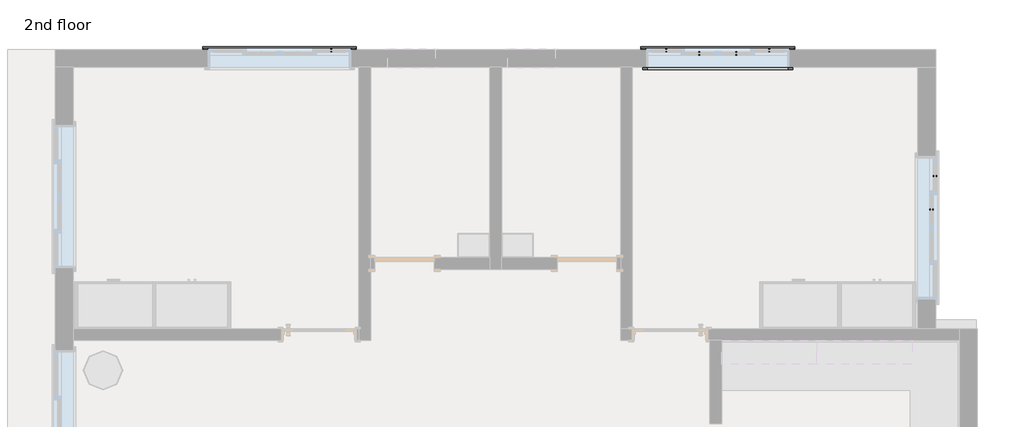
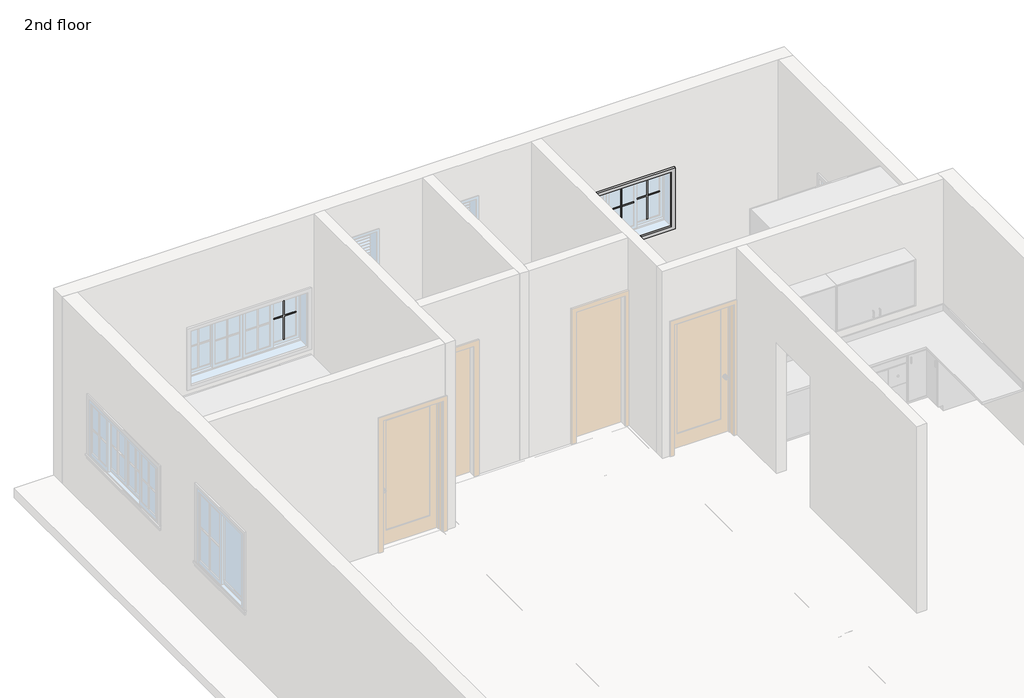
# One storey, part 4 of 4: 10 proxies.
"""IFC4 building model written with IfcOpenShell, lengths in millimetres."""

from ifc_helpers import new_model, si_unit, origin, place, context, project, spatial, transform, mapped, element, save
from components import muntin_pattern_2x2_muntin_pattern_2x2_31a16349, trim_window_exterior_flat_with_sill_3c945769, trim_window_interior_flat_picture_frame_0edfbaa2

model = new_model("IFC4")

# Units and contexts
model_context = context("Model", 3, world=origin())
ifc_project = project(units=[si_unit("LENGTHUNIT", "METRE", prefix="MILLI")], contexts=[model_context])

# Site, building, storey
site = spatial("IfcSite", under=ifc_project)
building = spatial("IfcBuilding", under=site)
storey = spatial("IfcBuildingStorey", under=building, Name="2nd floor", Elevation=7010.4)

# Proxies
placement = place(None, origin())
muntin_pattern_2x2_muntin_pattern_2x2_shape = muntin_pattern_2x2_muntin_pattern_2x2_31a16349(model_context)
element("IfcBuildingElementProxy", 1, Name="Muntin Pattern_2x2 : Muntin Pattern_2x2", ObjectType="Muntin Pattern_2x2 : Muntin Pattern_2x2", at=placement, inside=storey, context=model_context, shape_type="MappedRepresentation", body=[
    mapped(muntin_pattern_2x2_muntin_pattern_2x2_shape, transform((-9111.6124084, 10171.2711804, 8007.35), x_axis=(1.0, 0.0, 0.0), y_axis=(0.0, 1.0, 0.0), z_axis=(0.0, 0.0, 1.0))),
])
element("IfcBuildingElementProxy", 2, Name="Muntin Pattern_2x2 : Muntin Pattern_2x2", ObjectType="Muntin Pattern_2x2 : Muntin Pattern_2x2", at=placement, inside=storey, context=model_context, shape_type="MappedRepresentation", body=[
    mapped(muntin_pattern_2x2_muntin_pattern_2x2_shape, transform((-1374.1374084, 8555.1961804, 8007.35), x_axis=(0.0, -1.0, 0.0), y_axis=(1.0, 0.0, 0.0), z_axis=(0.0, 0.0, 1.0))),
])
element("IfcBuildingElementProxy", 3, Name="Muntin Pattern_2x2 : Muntin Pattern_2x2", ObjectType="Muntin Pattern_2x2 : Muntin Pattern_2x2", at=placement, inside=storey, context=model_context, shape_type="MappedRepresentation", body=[
    mapped(muntin_pattern_2x2_muntin_pattern_2x2_shape, transform((-1418.5874084, 8129.7461804, 8007.35), x_axis=(0.0, -1.0, 0.0), y_axis=(1.0, 0.0, 0.0), z_axis=(0.0, 0.0, 1.0))),
])
element("IfcBuildingElementProxy", 4, Name="Muntin Pattern_2x2 : Muntin Pattern_2x2", ObjectType="Muntin Pattern_2x2 : Muntin Pattern_2x2", at=placement, inside=storey, context=model_context, shape_type="MappedRepresentation", body=[
    mapped(muntin_pattern_2x2_muntin_pattern_2x2_shape, transform((-4819.0124084, 10171.2711804, 8007.35), x_axis=(1.0, 0.0, 0.0), y_axis=(0.0, 1.0, 0.0), z_axis=(0.0, 0.0, 1.0))),
])
element("IfcBuildingElementProxy", 5, Name="Muntin Pattern_2x2 : Muntin Pattern_2x2", ObjectType="Muntin Pattern_2x2 : Muntin Pattern_2x2", at=placement, inside=storey, context=model_context, shape_type="MappedRepresentation", body=[
    mapped(muntin_pattern_2x2_muntin_pattern_2x2_shape, transform((-4393.5624084, 10126.8211804, 8007.35), x_axis=(1.0, 0.0, 0.0), y_axis=(0.0, 1.0, 0.0), z_axis=(0.0, 0.0, 1.0))),
])
element("IfcBuildingElementProxy", 6, Name="Muntin Pattern_2x2 : Muntin Pattern_2x2", ObjectType="Muntin Pattern_2x2 : Muntin Pattern_2x2", at=placement, inside=storey, context=model_context, shape_type="MappedRepresentation", body=[
    mapped(muntin_pattern_2x2_muntin_pattern_2x2_shape, transform((-3923.6624084, 10126.8211804, 8007.35), x_axis=(1.0, 0.0, 0.0), y_axis=(0.0, 1.0, 0.0), z_axis=(0.0, 0.0, 1.0))),
])
element("IfcBuildingElementProxy", 7, Name="Muntin Pattern_2x2 : Muntin Pattern_2x2", ObjectType="Muntin Pattern_2x2 : Muntin Pattern_2x2", at=placement, inside=storey, context=model_context, shape_type="MappedRepresentation", body=[
    mapped(muntin_pattern_2x2_muntin_pattern_2x2_shape, transform((-3498.2124084, 10171.2711804, 8007.35), x_axis=(1.0, 0.0, 0.0), y_axis=(0.0, 1.0, 0.0), z_axis=(0.0, 0.0, 1.0))),
])
trim_window_exterior_flat_with_sill_shape = trim_window_exterior_flat_with_sill_3c945769(model_context)
element("IfcBuildingElementProxy", 8, Name="Trim-Window-Exterior-Flat : with Sill", ObjectType="Trim-Window-Exterior-Flat : with Sill", at=placement, inside=storey, context=model_context, shape_type="MappedRepresentation", body=[
    mapped(trim_window_exterior_flat_with_sill_shape, transform((-9772.0124084, 10180.7961804, 8839.2), x_axis=(-1.0, 0.0, 0.0), y_axis=(0.0, 0.0, 1.0), z_axis=(0.0, 1.0, 0.0))),
])
element("IfcBuildingElementProxy", 9, Name="Trim-Window-Exterior-Flat : with Sill", ObjectType="Trim-Window-Exterior-Flat : with Sill", at=placement, inside=storey, context=model_context, shape_type="MappedRepresentation", body=[
    mapped(trim_window_exterior_flat_with_sill_shape, transform((-4158.6124084, 10180.7961804, 8839.2), x_axis=(-1.0, 0.0, 0.0), y_axis=(0.0, 0.0, 1.0), z_axis=(0.0, 1.0, 0.0))),
])
trim_window_interior_flat_picture_frame_shape = trim_window_interior_flat_picture_frame_0edfbaa2(model_context)
element("IfcBuildingElementProxy", 10, Name="Trim-Window-Interior-Flat : Picture Frame", ObjectType="Trim-Window-Interior-Flat : Picture Frame", at=placement, inside=storey, context=model_context, shape_type="MappedRepresentation", body=[
    mapped(trim_window_interior_flat_picture_frame_shape, transform((-4158.6124084, 9952.1961804, 8839.2), x_axis=(1.0, 0.0, 0.0), y_axis=(0.0, 0.0, 1.0), z_axis=(0.0, -1.0, 0.0))),
])

save(model, "model.ifc")

# Revit data of these elements
# Type "Muntin Pattern_2x2 : Muntin Pattern_2x2"
#   Width [instance default] = 4' - 0"
#   Thickness = 0' - 0 1/2"
#   Height [instance default] = 4' - 0"
#   Distance = 0' - 0 3/4"
#   Interior Material [instance default] = none
#   Exterior Material [instance default] = none
#   Default Elevation = 0
# Type "Trim-Window-Exterior-Flat : with Sill"
#   Trim Width = 0' - 2 1/4"
#   Trim Thickness_Picture Frame = 0' - 1 1/4"
#   Trim Thickness_with Sill = 0' - 0 3/4"
#   Sill Thickness = 0' - 1 1/4"
#   Opening Width [instance default] = 2' - 0"
#   Opening Height [instance default] = 3' - 0"
#   Default Elevation = 4' - 0"
#   Sill = yes
#   Picture Frame = no
#   Trim Material [instance default] = none
# Type "Trim-Window-Interior-Flat : Picture Frame"
#   Trim Thickness_Picture Frame = 0' - 1 1/4"
#   Trim Width = 0' - 2 1/4"
#   Trim Thickness_with Sill = 0' - 0 3/4"
#   Sill Thickness = 0' - 1 1/4"
#   Opening Width [instance default] = 2' - 0"
#   Opening Height [instance default] = 3' - 0"
#   Default Elevation = 4' - 0"
#   Sill = no
#   Picture Frame = yes
#   Trim Material [instance default] = none
# Elements 1, 2, 3, 4, 5, 6, 7 (IfcBuildingElementProxy, "Muntin Pattern_2x2 : Muntin Pattern_2x2")
#   Width = 1' - 3"
#   Height = 2' - 6 1/4"
#   Interior Material = Wood - Stained
#   Exterior Material = Clad - White
#   Phase Created = New Construction
#   Materials on its faces: "Clad - White", "Wood - Stained"
# Elements 8, 9 (IfcBuildingElementProxy, "Trim-Window-Exterior-Flat : with Sill")
#   Opening Width = 6' - 0"
#   Opening Height = 3' - 0"
#   Trim Material = Clad - White
#   Phase Created = New Construction
#   Materials on its faces: "Clad - White"
# Element 10 (IfcBuildingElementProxy, "Trim-Window-Interior-Flat : Picture Frame")
#   Opening Width = 6' - 0"
#   Opening Height = 3' - 0"
#   Trim Material = Wood - Stained
#   Phase Created = New Construction
#   Materials on its faces: "Wood - Stained"
# Materials
#   "Clad - White": class "Wood", colour RGB 242 242 238, transparency 0, Cost = 0
#   "Wood - Stained": class "Wood", colour RGB 224 178 126, transparency 0, Cost = 0
